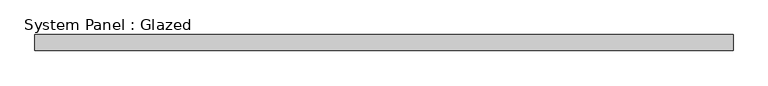
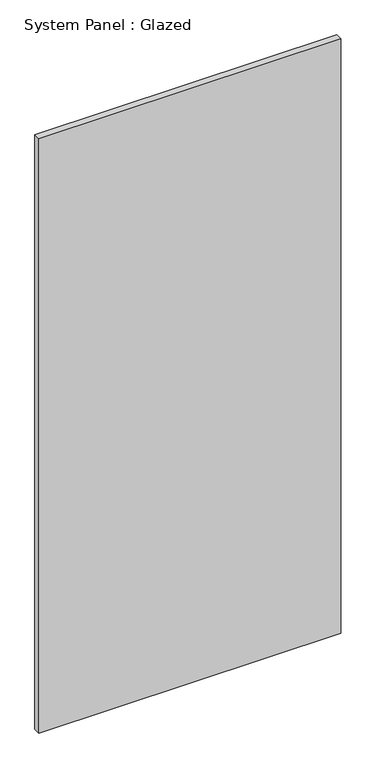
"""IFC4 building model written with IfcOpenShell, lengths in millimetres: plate geometry, System Panel : Glazed."""

from ifc_helpers import new_model, si_unit, origin, origin_with_axes, place, context, project, spatial, polyline, outline, extrude, source, transform, mapped, element, save


def system_panel_glazed_72e6272a(model_context):
    return source(origin(), model_context, "Body", "SweptSolid", [
        extrude(outline(polyline([(555.625, 19.05), (-555.625, 19.05), (-555.625, 44.45), (555.625, 44.45), (555.625, 19.05)])), origin_with_axes(), (0.0, 0.0, 1.0), 2311.4),
    ])


if __name__ == "__main__":
    model = new_model("IFC4")
    model_context = context("Model", 3, world=origin())
    ifc_project = project(units=[si_unit("LENGTHUNIT", "METRE", prefix="MILLI")], contexts=[model_context])
    site = spatial("IfcSite", under=ifc_project)
    building = spatial("IfcBuilding", under=site)
    placement = place(None, origin())
    system_panel_glazed_shape = system_panel_glazed_72e6272a(model_context)
    element("IfcPlate", 1, ObjectType="System Panel : Glazed", at=placement, inside=building, context=model_context, shape_type="MappedRepresentation", body=[
        mapped(system_panel_glazed_shape, transform((0.0, 0.0, 0.0), x_axis=(1.0, 0.0, 0.0), y_axis=(0.0, 1.0, 0.0), z_axis=(0.0, 0.0, 1.0))),
    ])
    save(model, "model.ifc")

# Revit data of these elements
# Type "System Panel : Glazed"
#   Construction Type Id = "GSP4R"
#   Analytic Construction = "1/8 in Pilkington single glazing"
#   Visual Light Transmittance = 0.9
#   Solar Heat Gain Coefficient = 0.86
#   Heat Transfer Coefficient (U) = 1.18115 BTU/(h·ft²·°F)
#   Define Thermal Properties by = 1
# Element 1 (IfcPlate, "System Panel : Glazed")
#   Materials on its faces: "Glass"
# Materials
#   "Glass": class "Glass", colour RGB 0 128 192, transparency 0.75, Description = "Soda Lime Glass", Cost = 0
